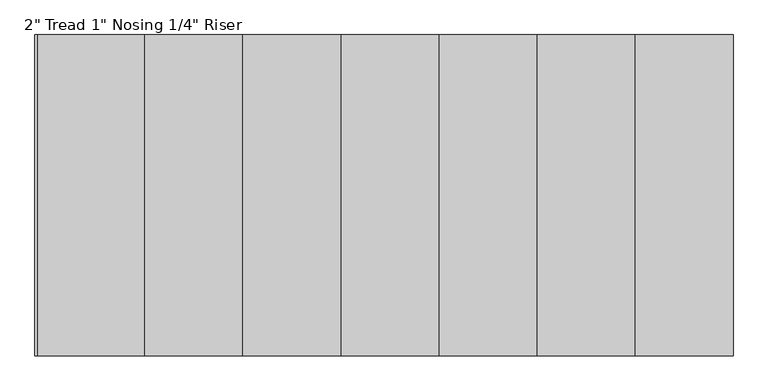
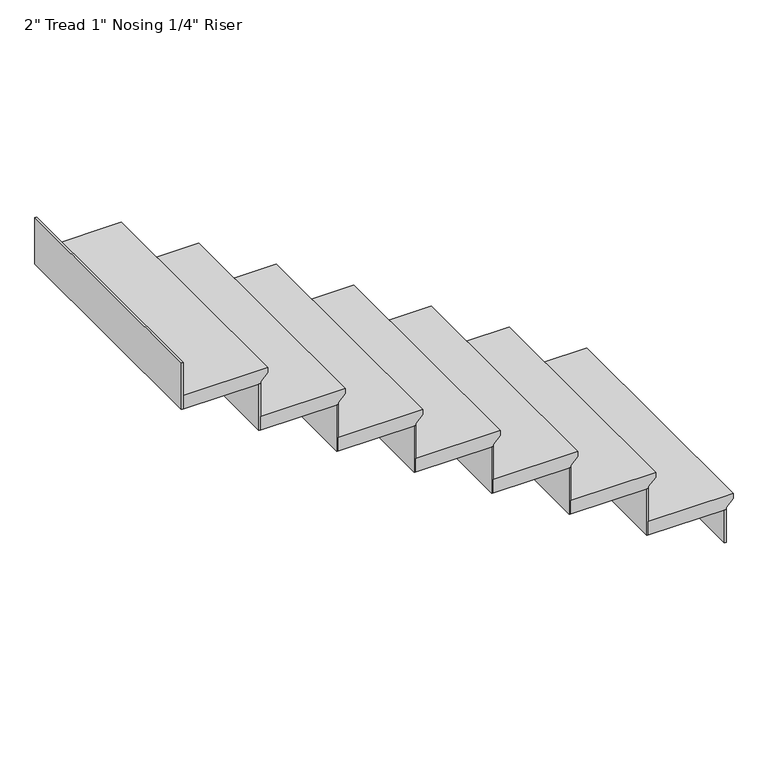
"""IFC4 building model written with IfcOpenShell, lengths in millimetres: stair flight geometry."""

from ifc_helpers import new_model, si_unit, origin, place, context, project, spatial, faceted_brep, source, transform, mapped, element, save


def stair_flight_1669251e(model_context):
    return source(origin(), model_context, "Body", "Brep", [
        faceted_brep([(31519.2316163, 9282.3980552, 768.35), (31519.2316163, 9282.3980552, 787.4), (31519.2316163, 8367.9980552, 787.4), (31519.2316163, 8367.9980552, 768.35), (31493.8316163, 9282.3980552, 742.95), (31493.8316163, 8367.9980552, 742.95), (31214.4316163, 9282.3980552, 787.4), (31214.4316163, 8367.9980552, 787.4), (31493.8316163, 8367.9980552, 736.6), (31214.4316163, 8367.9980552, 736.6), (31214.4316163, 9282.3980552, 736.6), (31493.8316163, 9282.3980552, 736.6)], [[[0, 1, 2, 3]], [[4, 0, 3, 5]], [[2, 1, 6, 7]], [[8, 9, 10, 11]], [[2, 7, 9, 8, 5, 3]], [[8, 11, 4, 5]], [[6, 1, 0, 4, 11, 10]], [[7, 6, 10, 9]]]),
        faceted_brep([(31493.8316163, 9282.3980552, 736.6), (31493.8316163, 9282.3980552, 609.6), (31487.4816163, 9282.3980552, 609.6), (31487.4816163, 9282.3980552, 736.6), (31493.8316163, 8367.9980552, 736.6), (31487.4816163, 8367.9980552, 736.6), (31487.4816163, 8367.9980552, 609.6), (31493.8316163, 8367.9980552, 609.6)], [[[0, 1, 2, 3]], [[4, 5, 6, 7]], [[1, 0, 4, 7]], [[2, 1, 7, 6]], [[3, 2, 6, 5]], [[0, 3, 5, 4]]]),
        faceted_brep([(31214.4316163, 9282.3980552, 914.4), (31214.4316163, 9282.3980552, 736.6), (31208.0816163, 9282.3980552, 736.6), (31208.0816163, 9282.3980552, 914.4), (31214.4316163, 8367.9980552, 914.4), (31208.0816163, 8367.9980552, 914.4), (31208.0816163, 8367.9980552, 736.6), (31214.4316163, 8367.9980552, 736.6)], [[[0, 1, 2, 3]], [[4, 5, 6, 7]], [[1, 0, 4, 7]], [[2, 1, 7, 6]], [[3, 2, 6, 5]], [[0, 3, 5, 4]]]),
        faceted_brep([(31239.8316163, 8367.9980552, 965.2), (31239.8316163, 9282.3980552, 965.2), (30935.0316163, 9282.3980552, 965.2), (30935.0316163, 8367.9980552, 965.2), (31214.4316163, 8367.9980552, 914.4), (30935.0316163, 8367.9980552, 914.4), (30935.0316163, 9282.3980552, 914.4), (31214.4316163, 9282.3980552, 914.4), (31214.4316163, 8367.9980552, 920.75), (31239.8316163, 8367.9980552, 946.15), (31214.4316163, 9282.3980552, 920.75), (31239.8316163, 9282.3980552, 946.15)], [[[0, 1, 2, 3]], [[4, 5, 6, 7]], [[0, 3, 5, 4, 8, 9]], [[4, 7, 10, 8]], [[2, 1, 11, 10, 7, 6]], [[3, 2, 6, 5]], [[11, 1, 0, 9]], [[10, 11, 9, 8]]]),
        faceted_brep([(30935.0316163, 9282.3980552, 1092.2), (30935.0316163, 9282.3980552, 914.4), (30928.6816163, 9282.3980552, 914.4), (30928.6816163, 9282.3980552, 1092.2), (30935.0316163, 8367.9980552, 1092.2), (30928.6816163, 8367.9980552, 1092.2), (30928.6816163, 8367.9980552, 914.4), (30935.0316163, 8367.9980552, 914.4)], [[[0, 1, 2, 3]], [[4, 5, 6, 7]], [[1, 0, 4, 7]], [[2, 1, 7, 6]], [[3, 2, 6, 5]], [[0, 3, 5, 4]]]),
        faceted_brep([(30960.4316163, 8367.9980552, 1143.0), (30960.4316163, 9282.3980552, 1143.0), (30655.6316163, 9282.3980552, 1143.0), (30655.6316163, 8367.9980552, 1143.0), (30935.0316163, 8367.9980552, 1092.2), (30655.6316163, 8367.9980552, 1092.2), (30655.6316163, 9282.3980552, 1092.2), (30935.0316163, 9282.3980552, 1092.2), (30935.0316163, 8367.9980552, 1098.55), (30960.4316163, 8367.9980552, 1123.95), (30935.0316163, 9282.3980552, 1098.55), (30960.4316163, 9282.3980552, 1123.95)], [[[0, 1, 2, 3]], [[4, 5, 6, 7]], [[0, 3, 5, 4, 8, 9]], [[4, 7, 10, 8]], [[2, 1, 11, 10, 7, 6]], [[3, 2, 6, 5]], [[11, 1, 0, 9]], [[10, 11, 9, 8]]]),
        faceted_brep([(30655.6316163, 9282.3980552, 1270.0), (30655.6316163, 9282.3980552, 1092.2), (30649.2816163, 9282.3980552, 1092.2), (30649.2816163, 9282.3980552, 1270.0), (30655.6316163, 8367.9980552, 1270.0), (30649.2816163, 8367.9980552, 1270.0), (30649.2816163, 8367.9980552, 1092.2), (30655.6316163, 8367.9980552, 1092.2)], [[[0, 1, 2, 3]], [[4, 5, 6, 7]], [[1, 0, 4, 7]], [[2, 1, 7, 6]], [[3, 2, 6, 5]], [[0, 3, 5, 4]]]),
        faceted_brep([(30681.0316163, 8367.9980552, 1320.8), (30681.0316163, 9282.3980552, 1320.8), (30376.2316163, 9282.3980552, 1320.8), (30376.2316163, 8367.9980552, 1320.8), (30655.6316163, 8367.9980552, 1270.0), (30376.2316163, 8367.9980552, 1270.0), (30376.2316163, 9282.3980552, 1270.0), (30655.6316163, 9282.3980552, 1270.0), (30655.6316163, 8367.9980552, 1276.35), (30681.0316163, 8367.9980552, 1301.75), (30655.6316163, 9282.3980552, 1276.35), (30681.0316163, 9282.3980552, 1301.75)], [[[0, 1, 2, 3]], [[4, 5, 6, 7]], [[0, 3, 5, 4, 8, 9]], [[4, 7, 10, 8]], [[2, 1, 11, 10, 7, 6]], [[3, 2, 6, 5]], [[11, 1, 0, 9]], [[10, 11, 9, 8]]]),
        faceted_brep([(30376.2316163, 9282.3980552, 1447.8), (30376.2316163, 9282.3980552, 1270.0), (30369.8816163, 9282.3980552, 1270.0), (30369.8816163, 9282.3980552, 1447.8), (30376.2316163, 8367.9980552, 1447.8), (30369.8816163, 8367.9980552, 1447.8), (30369.8816163, 8367.9980552, 1270.0), (30376.2316163, 8367.9980552, 1270.0)], [[[0, 1, 2, 3]], [[4, 5, 6, 7]], [[1, 0, 4, 7]], [[2, 1, 7, 6]], [[3, 2, 6, 5]], [[0, 3, 5, 4]]]),
        faceted_brep([(30401.6316163, 8367.9980552, 1498.6), (30401.6316163, 9282.3980552, 1498.6), (30096.8316163, 9282.3980552, 1498.6), (30096.8316163, 8367.9980552, 1498.6), (30376.2316163, 8367.9980552, 1447.8), (30096.8316163, 8367.9980552, 1447.8), (30096.8316163, 9282.3980552, 1447.8), (30376.2316163, 9282.3980552, 1447.8), (30376.2316163, 8367.9980552, 1454.15), (30401.6316163, 8367.9980552, 1479.55), (30376.2316163, 9282.3980552, 1454.15), (30401.6316163, 9282.3980552, 1479.55)], [[[0, 1, 2, 3]], [[4, 5, 6, 7]], [[0, 3, 5, 4, 8, 9]], [[4, 7, 10, 8]], [[2, 1, 11, 10, 7, 6]], [[3, 2, 6, 5]], [[11, 1, 0, 9]], [[10, 11, 9, 8]]]),
        faceted_brep([(30096.8316163, 9282.3980552, 1625.6), (30096.8316163, 9282.3980552, 1447.8), (30090.4816163, 9282.3980552, 1447.8), (30090.4816163, 9282.3980552, 1625.6), (30096.8316163, 8367.9980552, 1625.6), (30090.4816163, 8367.9980552, 1625.6), (30090.4816163, 8367.9980552, 1447.8), (30096.8316163, 8367.9980552, 1447.8)], [[[0, 1, 2, 3]], [[4, 5, 6, 7]], [[1, 0, 4, 7]], [[2, 1, 7, 6]], [[3, 2, 6, 5]], [[0, 3, 5, 4]]]),
        faceted_brep([(30122.2316163, 8367.9980552, 1676.4), (30122.2316163, 9282.3980552, 1676.4), (29817.4316163, 9282.3980552, 1676.4), (29817.4316163, 8367.9980552, 1676.4), (30096.8316163, 8367.9980552, 1625.6), (29817.4316163, 8367.9980552, 1625.6), (29817.4316163, 9282.3980552, 1625.6), (30096.8316163, 9282.3980552, 1625.6), (30096.8316163, 8367.9980552, 1631.95), (30122.2316163, 8367.9980552, 1657.35), (30096.8316163, 9282.3980552, 1631.95), (30122.2316163, 9282.3980552, 1657.35)], [[[0, 1, 2, 3]], [[4, 5, 6, 7]], [[0, 3, 5, 4, 8, 9]], [[4, 7, 10, 8]], [[2, 1, 11, 10, 7, 6]], [[3, 2, 6, 5]], [[11, 1, 0, 9]], [[10, 11, 9, 8]]]),
        faceted_brep([(29538.0316163, 9282.3980552, 1981.2), (29538.0316163, 9282.3980552, 1803.4), (29531.6816163, 9282.3980552, 1803.4), (29531.6816163, 9282.3980552, 1981.2), (29538.0316163, 8367.9980552, 1981.2), (29531.6816163, 8367.9980552, 1981.2), (29531.6816163, 8367.9980552, 1803.4), (29538.0316163, 8367.9980552, 1803.4)], [[[0, 1, 2, 3]], [[4, 5, 6, 7]], [[1, 0, 4, 7]], [[2, 1, 7, 6]], [[3, 2, 6, 5]], [[0, 3, 5, 4]]]),
        faceted_brep([(29817.4316163, 9282.3980552, 1803.4), (29817.4316163, 9282.3980552, 1625.6), (29811.0816163, 9282.3980552, 1625.6), (29811.0816163, 9282.3980552, 1803.4), (29817.4316163, 8367.9980552, 1803.4), (29811.0816163, 8367.9980552, 1803.4), (29811.0816163, 8367.9980552, 1625.6), (29817.4316163, 8367.9980552, 1625.6)], [[[0, 1, 2, 3]], [[4, 5, 6, 7]], [[1, 0, 4, 7]], [[2, 1, 7, 6]], [[3, 2, 6, 5]], [[0, 3, 5, 4]]]),
        faceted_brep([(29842.8316163, 8367.9980552, 1854.2), (29842.8316163, 9282.3980552, 1854.2), (29563.4316163, 9282.3980552, 1854.2), (29538.0316163, 9282.3980552, 1854.2), (29538.0316163, 8367.9980552, 1854.2), (29817.4316163, 8367.9980552, 1803.4), (29538.0316163, 8367.9980552, 1803.4), (29538.0316163, 9282.3980552, 1803.4), (29563.4316163, 9282.3980552, 1803.4), (29817.4316163, 9282.3980552, 1803.4), (29817.4316163, 8367.9980552, 1809.75), (29842.8316163, 8367.9980552, 1835.15), (29817.4316163, 9282.3980552, 1809.75), (29842.8316163, 9282.3980552, 1835.15)], [[[0, 1, 2, 3, 4]], [[5, 6, 7, 8, 9]], [[0, 4, 6, 5, 10, 11]], [[5, 9, 12, 10]], [[2, 1, 13, 12, 9, 8]], [[3, 2, 8, 7]], [[4, 3, 7, 6]], [[13, 1, 0, 11]], [[12, 13, 11, 10]]]),
    ])


if __name__ == "__main__":
    model = new_model("IFC4")
    model_context = context("Model", 3, world=origin())
    ifc_project = project(units=[si_unit("LENGTHUNIT", "METRE", prefix="MILLI")], contexts=[model_context])
    site = spatial("IfcSite", under=ifc_project)
    building = spatial("IfcBuilding", under=site)
    placement = place(None, origin())
    stair_flight_shape = stair_flight_1669251e(model_context)
    element("IfcStairFlight", 1, ObjectType="2\" Tread 1\" Nosing 1/4\" Riser", at=placement, inside=building, context=model_context, shape_type="MappedRepresentation", body=[
        mapped(stair_flight_shape, transform((0.0, 0.0, 0.0), x_axis=(1.0, 0.0, 0.0), y_axis=(0.0, 1.0, 0.0), z_axis=(0.0, 0.0, 1.0))),
    ])
    save(model, "model.ifc")
